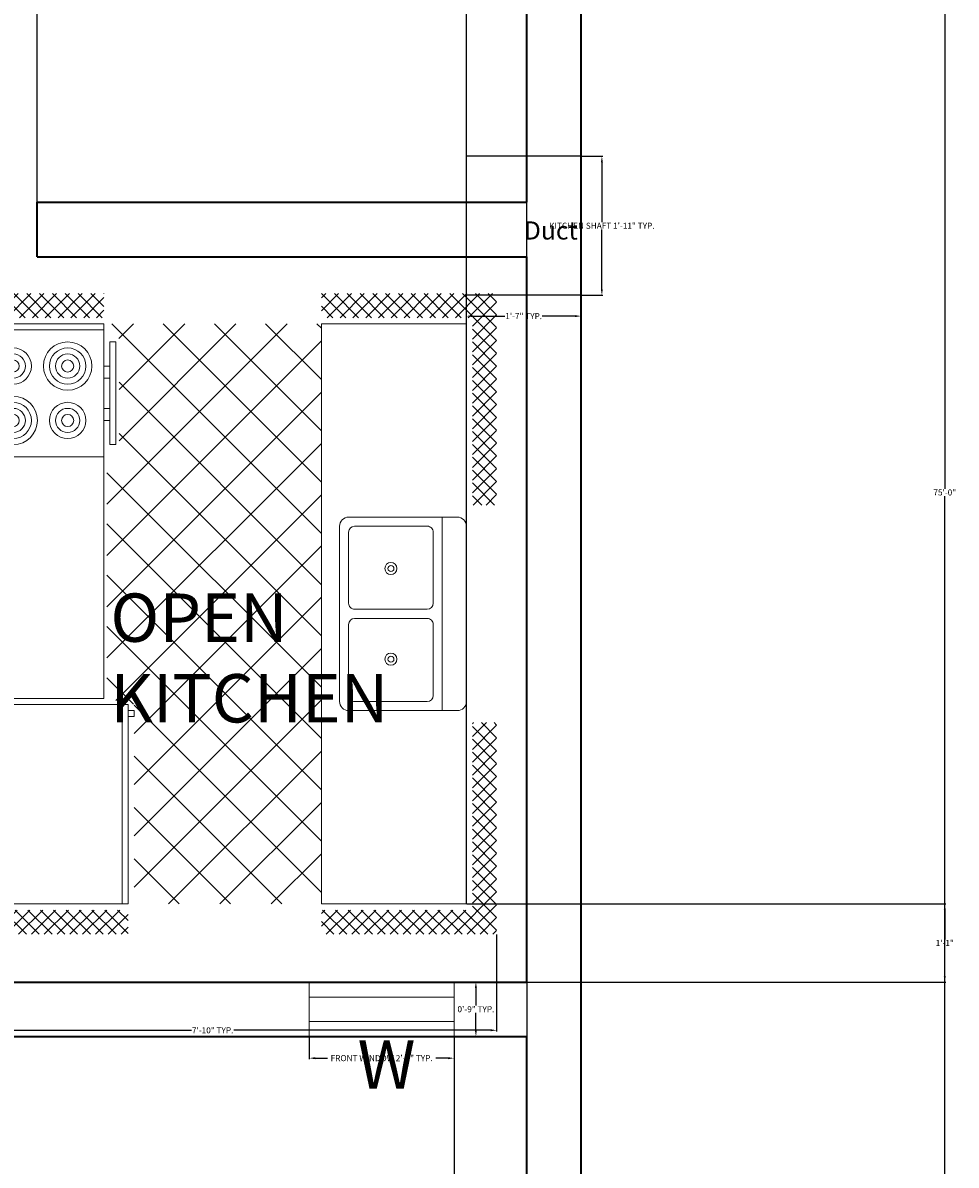
# Model space of a CAD drawing. Units: inches. Extents: x 371 to 1095, y -45 to 1219.
# Tile 12 of 18: x 940 to 1095, y 421 to 610. Entities that reach past the tile are written whole.
import ezdxf

# ---------------------------------------------------------------- set-up
doc = ezdxf.new("R2010")
doc.units = ezdxf.units.IN
doc.header["$MEASUREMENT"] = 0
for name, color, linetype, lineweight in [('A-ANNO-DIMS', 2, 'Continuous', 18), ('A-ANNO-TEXT', 7, 'Continuous', 18), ('A-AREA-IDEN', 7, 'Continuous', 18), ('A-FLOR-FIXT', 9, 'Continuous', 18), ('A-FLOR-SHFT', 7, 'Continuous', 25), ('A-GLAZ', 4, 'Continuous', 18), ('A-WALL', 40, 'Continuous', 35), ('C-SITE-WALL', 40, 'Continuous', 35)]:
    doc.layers.add(name, color=color, linetype=linetype, lineweight=lineweight)
doc.styles.get("Standard").update_dxf_attribs({"font": 'arial.ttf'})
doc.dimstyles.get("Standard").update_dxf_attribs({"dimtxt": 1, "dimasz": 1, "dimexe": 0.18, "dimexo": 0.0625, "dimgap": 0.09, "dimtad": 0, "dimtih": 1, "dimtoh": 1, "dimdec": 0, "dimzin": 0, "dimdsep": 46, "dimlunit": 3, "dimtxsty": 'Standard', "dimcen": 0.09, "dimadec": 0, "dimazin": 0, "dimtfac": 1, "dimtdec": 0, "dimtofl": 0, "dimtmove": 0, "dimatfit": 3, "dimfxl": 1, "dimtolj": 1, "dimtzin": 0, "dimarcsym": 0})

# ---------------------------------------------------------------- blocks, each defined once
blk = doc.blocks.new('Kitchen Layout - 7 x 8 ft')
for p, q in [((-5, 81.32), (2.68, 89)), ((-5, 83.44), (0.56, 89)), ((-5, 85.56), (-1.56, 89)), ((-5, 87.68), (-3.68, 89)), ((-1, 84.97), (-5, 88.97)), ((1.09, 85), (-2.91, 89)), ((3.21, 85), (-0.79, 89)), ((0.81, 85), (4.81, 89)), ((5.34, 85), (1.34, 89)), ((2.93, 85), (6.93, 89)), ((7.46, 85), (3.46, 89)), ((5.05, 85), (9.05, 89)), ((9.58, 85), (5.58, 89)), ((7.17, 85), (11.17, 89)), ((11.7, 85), (7.7, 89)), ((9.29, 85), (13.29, 89)), ((13.82, 85), (9.82, 89)), ((11.41, 85), (15.41, 89)), ((15.94, 85), (11.94, 89)), ((13.53, 85), (17.53, 89)), ((18.06, 85), (14.06, 89)), ((15.65, 85), (19.65, 89)), ((20.18, 85), (16.18, 89)), ((17.78, 85), (21.78, 89)), ((22.31, 85), (18.31, 89)), ((19.9, 85), (23.9, 89)), ((24.43, 85), (20.43, 89)), ((22.02, 85), (26.02, 89)), ((26.55, 85), (22.55, 89)), ((24.14, 85), (28.14, 89)), ((28.67, 85), (24.67, 89)), ((26.26, 85), (30.26, 89)), ((30.79, 85), (26.79, 89)), ((28.38, 85), (32.38, 89)), ((32.91, 85), (28.91, 89)), ((30.5, 85), (34.5, 89)), ((35.03, 85), (31.03, 89)), ((32.63, 85), (36.63, 89)), ((37.16, 85), (33.16, 89)), ((34.75, 85), (38.75, 89)), ((39.28, 85), (35.28, 89)), ((36.87, 85), (40.87, 89)), ((41.4, 85), (37.4, 89)), ((38.99, 85), (42.99, 89)), ((43.52, 85), (39.52, 89)), ((41.11, 85), (45.11, 89)), ((45.64, 85), (41.64, 89)), ((43.23, 85), (47.23, 89)), ((47.76, 85), (43.76, 89)), ((45.35, 85), (49.35, 89)), ((49.88, 85), (45.88, 89)), ((47.47, 85), (51.47, 89)), ((52, 85), (48, 89)), ((49.6, 85), (53.6, 89)), ((54.13, 85), (50.13, 89)), ((51.72, 85), (55.72, 89)), ((56.25, 85), (52.25, 89)), ((53.84, 85), (57.84, 89)), ((58.37, 85), (54.37, 89)), ((55.96, 85), (59.96, 89)), ((60.49, 85), (56.49, 89)), ((58.08, 85), (62.08, 89)), ((62.61, 85), (58.61, 89)), ((60.2, 85), (64.2, 89)), ((64.73, 85), (60.73, 89)), ((62.32, 85), (66.32, 89)), ((66.85, 85), (62.85, 89)), ((64.45, 85), (68.45, 89)), ((68.97, 85), (64.97, 89)), ((66.57, 85), (70.57, 89)), ((71.1, 85), (67.1, 89)), ((68.69, 85), (72.69, 89)), ((73.22, 85), (69.22, 89)), ((70.81, 85), (74.81, 89)), ((75.34, 85), (71.34, 89)), ((72.93, 85), (76.93, 89)), ((77.46, 85), (73.46, 89)), ((75.05, 85), (79.05, 89)), ((79.58, 85), (75.58, 89)), ((77.17, 85), (81.17, 89)), ((81.7, 85), (77.7, 89)), ((79.29, 85), (83.29, 89)), ((83.82, 85), (79.82, 89)), ((81.42, 85), (85.42, 89)), ((85.95, 85), (81.95, 89)), ((83.54, 85), (87.54, 89)), ((88.07, 85), (84.07, 89)), ((85.66, 85), (89.66, 89)), ((90.19, 85), (86.19, 89)), ((87.78, 85), (91.78, 89)), ((92.31, 85), (88.31, 89)), ((89.9, 85), (93.9, 89)), ((94.43, 85), (90.43, 89)), ((92.02, 85), (96.02, 89)), ((96.55, 85), (92.55, 89)), ((94.14, 85), (98.14, 89)), ((101, 82.67), (94.67, 89)), ((96.27, 85), (100.27, 89)), ((101, 84.79), (96.79, 89)), ((101, 86.92), (98.92, 89)), ((97, 83.61), (101, 87.61)), ((-1, 82.85), (-5, 86.85)), ((97, 81.49), (101, 85.49)), ((-1, 80.73), (-5, 84.73)), ((-5, 79.19), (-1, 83.19)), ((34, 84), (96, 84)), ((34, 60), (34, 84)), ((96, 84), (96, 60)), ((101, 80.55), (97, 84.55)), ((97, 79.37), (101, 83.37)), ((-1, 78.61), (-5, 82.61)), ((101, 78.43), (97, 82.43)), ((-5, 77.07), (-1, 81.07)), ((-1, 76.49), (-5, 80.49)), ((74, 81), (95, 81)), ((97, 77.25), (101, 81.25)), ((101, 76.31), (97, 80.31)), ((-5, 74.95), (-1, 78.95)), ((-1, 74.36), (-5, 78.36)), ((97, 75.13), (101, 79.13)), ((101, 74.19), (97, 78.19)), ((-5, 72.83), (-1, 76.83)), ((-1, 72.24), (-5, 76.24)), ((97, 73.01), (101, 77.01)), ((101, 72.07), (97, 76.07)), ((-5, 70.71), (-1, 74.71)), ((-1, 70.12), (-5, 74.12)), ((97, 70.89), (101, 74.89)), ((101, 69.95), (97, 73.95)), ((-5, 68.59), (-1, 72.59)), ((-1, 68), (-5, 72)), ((97, 68.76), (101, 72.76)), ((101, 67.82), (97, 71.82)), ((-5, 66.47), (-1, 70.47)), ((97, 66.64), (101, 70.64)), ((-1, 65.88), (-5, 69.88)), ((-5, 64.35), (-1, 68.35)), ((101, 65.7), (97, 69.7)), ((97, 64.52), (101, 68.52)), ((-1, 63.76), (-5, 67.76)), ((-5, 62.22), (-1, 66.22)), ((101, 63.58), (97, 67.58)), ((97, 62.4), (101, 66.4)), ((-1, 61.64), (-5, 65.64)), ((101, 61.46), (97, 65.46)), ((97, 60.28), (101, 64.28)), ((-5, 60.1), (-1, 64.1)), ((-1, 59.52), (-5, 63.52)), ((100.34, 60), (97, 63.34)), ((-5, 57.98), (-1, 61.98)), ((-1, 57.39), (-5, 61.39)), ((98.22, 60), (97, 61.22)), ((98.84, 60), (101, 62.16)), ((-1.73, 56), (-5, 59.27)), ((-4.86, 56), (-1, 59.86)), ((10.4, 24), (45.9, 59.5)), ((18.88, 24), (54.38, 59.5)), ((27.37, 24), (62.87, 59.5)), ((33.03, 55.11), (37.41, 59.5)), ((96, 60), (34, 60)), ((35.85, 24), (71.35, 59.5)), ((76.2, 24), (40.7, 59.5)), ((84.68, 24), (49.18, 59.5)), ((93.17, 24), (57.67, 59.5)), ((61.31, 24), (96, 58.69)), ((96, 29.65), (66.15, 59.5)), ((80, 60), (80, 59)), ((82, 59), (82, 60)), ((87, 59), (87, 60)), ((89, 60), (89, 59)), ((100.96, 60), (101, 60.04)), ((-3.85, 56), (-5, 57.15)), ((-2.74, 56), (-1, 57.74)), ((0, 57), (33, 57)), ((67.71, 24), (33.68, 58.04)), ((44.34, 24), (77.84, 57.5)), ((52.82, 24), (86.32, 57.5)), ((96, 38.14), (76.64, 57.5)), ((96, 46.63), (85.13, 57.5)), ((96, 55.11), (93.57, 57.54)), ((0, 30.57), (24.43, 55)), ((0, 39.06), (15.94, 55)), ((0, 47.54), (7.46, 55)), ((1.91, 24), (32.91, 55)), ((33.77, 24), (2.77, 55)), ((42.26, 24), (11.26, 55)), ((50.74, 24), (19.74, 55)), ((59.23, 24), (28.23, 55)), ((31, 55), (31, 56)), ((32, 55), (31, 55)), ((32, 56), (32, 55)), ((25.29, 24), (0, 49.29)), ((69.79, 24), (96, 50.21)), ((78.28, 24), (96, 41.72)), ((16.8, 24), (0, 40.8)), ((8.32, 24), (0, 32.32)), ((86.76, 24), (96, 33.24)), ((95.25, 24), (96, 24.75)), ((-5, 21.92), (-2.92, 24)), ((-5, 19.8), (-1, 23.8)), ((-1, 19.21), (-5, 23.21)), ((-1, 21.33), (-3.67, 24)), ((-1, 23.45), (-1.55, 24)), ((0, 24), (96, 24)), ((0, 0), (0, 24)), ((96, 24), (96, 0)), ((97, 22.1), (98.9, 24)), ((97, 19.97), (101, 23.97)), ((101, 19.03), (97, 23.03)), ((101, 21.16), (98.16, 24)), ((101, 23.28), (100.28, 24)), ((-5, 17.68), (-1, 21.68)), ((-1, 17.09), (-5, 21.09)), ((97, 17.85), (101, 21.85)), ((101, 16.91), (97, 20.91)), ((-5, 15.55), (-1, 19.55)), ((-1, 14.97), (-5, 18.97)), ((97, 15.73), (101, 19.73)), ((-5, 13.43), (-1, 17.43)), ((47.25, 6.5), (47.25, 18.5)), ((48.75, 18.5), (48.75, 6.5)), ((101, 14.79), (97, 18.79)), ((97, 13.61), (101, 17.61)), ((-1, 12.85), (-5, 16.85)), ((-5, 11.31), (-1, 15.31)), ((101, 12.67), (97, 16.67)), ((97, 11.49), (101, 15.49)), ((-1, 10.73), (-5, 14.73)), ((101, 10.55), (97, 14.55)), ((97, 9.37), (101, 13.37)), ((-5, 9.19), (-1, 13.19)), ((-1, 8.6), (-5, 12.6)), ((101, 8.43), (97, 12.43)), ((-5, 7.07), (-1, 11.07)), ((-1, 6.48), (-5, 10.48)), ((97, 7.25), (101, 11.25)), ((101, 6.31), (97, 10.31)), ((-5, 4.95), (-1, 8.95)), ((-1, 4.36), (-5, 8.36)), ((97, 5.12), (101, 9.12)), ((101, 4.18), (97, 8.18)), ((-5, 2.83), (-1, 6.83)), ((-1, 2.24), (-5, 6.24)), ((97, 3), (101, 7)), ((101, 2.06), (97, 6.06)), ((-5, 0.71), (-1, 4.71)), ((-1, 0.12), (-5, 4.12)), ((64, 4), (32, 4)), ((97, 0.88), (101, 4.88)), ((101, -0.06), (97, 3.94)), ((-5, -1.42), (-1, 2.58)), ((2, -5), (-5, 2)), ((93.24, -5), (101, 2.76)), ((-5, -3.54), (-1, 0.46)), ((96, 0), (0, 0)), ((95.36, -5), (101, 0.64)), ((101, -2.18), (97, 1.82)), ((-0.12, -5), (-5, -0.12)), ((-4.34, -5), (-0.34, -1)), ((-2.22, -5), (1.78, -1)), ((-0.1, -5), (3.9, -1)), ((4.12, -5), (0.12, -1)), ((2.02, -5), (6.02, -1)), ((6.24, -5), (2.24, -1)), ((4.14, -5), (8.14, -1)), ((8.36, -5), (4.36, -1)), ((6.27, -5), (10.27, -1)), ((10.48, -5), (6.48, -1)), ((8.39, -5), (12.39, -1)), ((12.6, -5), (8.6, -1)), ((10.51, -5), (14.51, -1)), ((14.73, -5), (10.73, -1)), ((12.63, -5), (16.63, -1)), ((16.85, -5), (12.85, -1)), ((14.75, -5), (18.75, -1)), ((18.97, -5), (14.97, -1)), ((16.87, -5), (20.87, -1)), ((21.09, -5), (17.09, -1)), ((18.99, -5), (22.99, -1)), ((23.21, -5), (19.21, -1)), ((21.11, -5), (25.11, -1)), ((25.33, -5), (21.33, -1)), ((23.24, -5), (27.24, -1)), ((27.45, -5), (23.45, -1)), ((25.36, -5), (29.36, -1)), ((29.57, -5), (25.57, -1)), ((30, -3.3), (27.7, -1)), ((30, -1.18), (29.82, -1)), ((66, -2.54), (67.54, -1)), ((66, -4.66), (69.66, -1)), ((69.88, -5), (66, -1.12)), ((67.78, -5), (71.78, -1)), ((72, -5), (68, -1)), ((69.9, -5), (73.9, -1)), ((74.12, -5), (70.12, -1)), ((72.03, -5), (76.03, -1)), ((76.24, -5), (72.24, -1)), ((74.15, -5), (78.15, -1)), ((78.36, -5), (74.36, -1)), ((76.27, -5), (80.27, -1)), ((80.49, -5), (76.49, -1)), ((78.39, -5), (82.39, -1)), ((82.61, -5), (78.61, -1)), ((80.51, -5), (84.51, -1)), ((84.73, -5), (80.73, -1)), ((82.63, -5), (86.63, -1)), ((86.85, -5), (82.85, -1)), ((84.75, -5), (88.75, -1)), ((88.97, -5), (84.97, -1)), ((86.88, -5), (90.88, -1)), ((91.09, -5), (87.09, -1)), ((89, -5), (93, -1)), ((93.21, -5), (89.21, -1)), ((91.12, -5), (95.12, -1)), ((95.34, -5), (91.34, -1)), ((97.46, -5), (93.46, -1)), ((99.58, -5), (95.58, -1)), ((101, -4.3), (97, -0.3)), ((97.48, -5), (101, -1.48)), ((-2.25, -5), (-5, -2.25)), ((27.48, -5), (30, -2.48)), ((67.76, -5), (66, -3.24)), ((99.6, -5), (101, -3.6)), ((-4.37, -5), (-5, -4.37)), ((29.6, -5), (30, -4.6))]:
    blk.add_line(p, q)
for points in [[(0, 56), (0, 84), (33, 84), (33, 56)], [(74, 60), (74, 84), (95, 84), (95, 60)], [(76, 58), (76, 59), (93, 59), (93, 58)]]:
    blk.add_lwpolyline(points, close=True)
for points in [[(33.5, 21), (62.5, 21)], [(32, 1.5), (32, 19.5)], [(34.5, 19.5), (46.25, 19.5)], [(49.75, 19.5), (61.5, 19.5)], [(64, 19.5), (64, 1.5)], [(33.5, 6.5), (33.5, 18.5)], [(62.5, 18.5), (62.5, 6.5)], [(46.25, 5.5), (34.5, 5.5)], [(61.5, 5.5), (49.75, 5.5)], [(62.5, 0), (33.5, 0)]]:
    blk.add_lwpolyline(points)
for centre, radius in [((80, 75), 4), ((80, 75), 3), ((89, 75), 3), ((80, 75), 2), ((80, 75), 1), ((89, 75), 2), ((89, 75), 1), ((89, 66), 4), ((80, 66), 3), ((89, 66), 3), ((80, 66), 2), ((80, 66), 1), ((89, 66), 2), ((89, 66), 1), ((40.5, 12.5), 1), ((55.5, 12.5), 1), ((40.5, 12.5), 0.5), ((55.5, 12.5), 0.5)]:
    blk.add_circle(centre, radius)
for centre, radius, start, end in [((33.5, 19.5), 1.5, 90, 180), ((62.5, 19.5), 1.5, 0, 90), ((34.5, 18.5), 1, 90, 180), ((46.25, 18.5), 1, 0, 90), ((49.75, 18.5), 1, 90, 180), ((61.5, 18.5), 1, 0, 90), ((34.5, 6.5), 1, 180, 270), ((46.25, 6.5), 1, 270, 0), ((49.75, 6.5), 1, 180, 270), ((61.5, 6.5), 1, 270, 0), ((33.5, 1.5), 1.5, 180, 270), ((62.5, 1.5), 1.5, 270, 0)]:
    blk.add_arc(centre, radius, start, end)
blk = doc.blocks.new('WIN-24-FRONT')
for p, q in [((0, 6.5), (24, 6.5)), ((0, 2.5), (24, 2.5))]:
    blk.add_line(p, q)
blk.add_lwpolyline([(0, 0), (24, 0), (24, 9), (0, 9)], close=True)
blk = doc.blocks.new('SHAFT-KITCHEN')
for p, q in [((19, 23), (0, 23)), ((0, 23), (0, 0)), ((19, 0), (19, 23)), ((19, 0), (0, 0))]:
    blk.add_line(p, q)
blk = doc.blocks.new('*D37')
at = {"layer": 'A-ANNO-DIMS', "color": 0, "lineweight": -2, "transparency": 16777216}
for p, q in [((924.84, 458.88), (924.84, 442.86)), ((1018.84, 458.88), (1018.84, 442.86)), ((925.84, 443.04), (968.31, 443.04)), ((1017.84, 443.04), (975.36, 443.04))]:
    blk.add_line(p, q, dxfattribs=at)
at = {"layer": 'A-ANNO-DIMS', "color": 0, "transparency": 16777216}
for points in [[(925.84, 443.21), (925.84, 442.88), (924.84, 443.04)], [(1017.84, 443.21), (1017.84, 442.88), (1018.84, 443.04)]]:
    blk.add_solid(points, dxfattribs=at)
at = {"layer": 'Defpoints', "color": 0, "transparency": 16777216}
for p in [(924.84, 458.94), (1018.84, 458.94), (924.84, 443.04)]:
    blk.add_point(p, dxfattribs=at)
at = {"layer": 'A-ANNO-DIMS', "color": 0, "transparency": 16777216, "insert": (971.84, 443.04), "char_height": 1, "attachment_point": 5}
blk.add_mtext('\\A1;7\'-10" TYP.', dxfattribs=at)
blk = doc.blocks.new('*D44')
at = {"layer": 'A-ANNO-DIMS', "color": 0, "lineweight": -2, "transparency": 16777216}
for p, q in [((987.81, 441.96), (987.81, 438.25)), ((1011.81, 441.96), (1011.81, 438.25)), ((988.81, 438.43), (990.84, 438.43)), ((1010.81, 438.43), (1008.78, 438.43))]:
    blk.add_line(p, q, dxfattribs=at)
at = {"layer": 'A-ANNO-DIMS', "color": 0, "transparency": 16777216}
for points in [[(988.81, 438.59), (988.81, 438.26), (987.81, 438.43)], [(1010.81, 438.59), (1010.81, 438.26), (1011.81, 438.43)]]:
    blk.add_solid(points, dxfattribs=at)
at = {"layer": 'Defpoints', "color": 0, "transparency": 16777216}
for p in [(987.81, 442.03), (1011.81, 442.03), (1011.81, 438.43)]:
    blk.add_point(p, dxfattribs=at)
at = {"layer": 'A-ANNO-DIMS', "color": 0, "transparency": 16777216, "insert": (999.81, 438.43), "char_height": 1, "attachment_point": 5}
blk.add_mtext('\\A1;FRONT WINDOW 2\'-0" TYP.', dxfattribs=at)
blk = doc.blocks.new('*D45')
at = {"layer": 'A-ANNO-DIMS', "color": 0, "lineweight": -2, "transparency": 16777216}
for p, q in [((1011.87, 451.03), (1015.59, 451.03)), ((1015.41, 450.03), (1015.41, 447.13)), ((1015.41, 443.03), (1015.41, 445.92)), ((1011.87, 442.03), (1015.59, 442.03))]:
    blk.add_line(p, q, dxfattribs=at)
at = {"layer": 'A-ANNO-DIMS', "color": 0, "transparency": 16777216}
for points in [[(1015.24, 450.03), (1015.57, 450.03), (1015.41, 451.03)], [(1015.24, 443.03), (1015.57, 443.03), (1015.41, 442.03)]]:
    blk.add_solid(points, dxfattribs=at)
at = {"layer": 'Defpoints', "color": 0, "transparency": 16777216}
for p in [(1011.81, 451.03), (1015.41, 451.03), (1011.81, 442.03)]:
    blk.add_point(p, dxfattribs=at)
at = {"layer": 'A-ANNO-DIMS', "color": 0, "transparency": 16777216, "insert": (1015.41, 446.53), "char_height": 1, "attachment_point": 5}
blk.add_mtext('\\A1;0\'-9" TYP.', dxfattribs=at)
blk = doc.blocks.new('*D48')
at = {"layer": 'A-ANNO-DIMS', "color": 0, "lineweight": -2, "transparency": 16777216}
for p, q in [((1032.87, 587.65), (1036.44, 587.65)), ((1036.26, 586.65), (1036.26, 576.76)), ((1036.26, 565.65), (1036.26, 575.55)), ((1032.87, 564.65), (1036.44, 564.65))]:
    blk.add_line(p, q, dxfattribs=at)
at = {"layer": 'A-ANNO-DIMS', "color": 0, "transparency": 16777216}
for points in [[(1036.09, 586.65), (1036.42, 586.65), (1036.26, 587.65)], [(1036.09, 565.65), (1036.42, 565.65), (1036.26, 564.65)]]:
    blk.add_solid(points, dxfattribs=at)
at = {"layer": 'Defpoints', "color": 0, "transparency": 16777216}
for p in [(1032.81, 587.65), (1036.26, 587.65), (1032.81, 564.65)]:
    blk.add_point(p, dxfattribs=at)
at = {"layer": 'A-ANNO-DIMS', "color": 0, "transparency": 16777216, "insert": (1036.26, 576.15), "char_height": 1, "attachment_point": 5}
blk.add_mtext('\\A1;KITCHEN SHAFT 1\'-11" TYP.', dxfattribs=at)
blk = doc.blocks.new('*D49')
at = {"layer": 'A-ANNO-DIMS', "color": 0, "lineweight": -2, "transparency": 16777216}
for p, q in [((1013.81, 564.59), (1013.81, 561.02)), ((1032.81, 564.59), (1032.81, 561.02)), ((1014.81, 561.2), (1020.22, 561.2)), ((1031.81, 561.2), (1026.4, 561.2))]:
    blk.add_line(p, q, dxfattribs=at)
at = {"layer": 'A-ANNO-DIMS', "color": 0, "transparency": 16777216}
for points in [[(1014.81, 561.37), (1014.81, 561.04), (1013.81, 561.2)], [(1031.81, 561.37), (1031.81, 561.04), (1032.81, 561.2)]]:
    blk.add_solid(points, dxfattribs=at)
at = {"layer": 'Defpoints', "color": 0, "transparency": 16777216}
for p in [(1013.81, 564.65), (1032.81, 564.65), (1032.81, 561.2)]:
    blk.add_point(p, dxfattribs=at)
at = {"layer": 'A-ANNO-DIMS', "color": 0, "transparency": 16777216, "insert": (1023.31, 561.2), "char_height": 1, "attachment_point": 5}
blk.add_mtext('\\A1;1\'-7" TYP.', dxfattribs=at)
blk = doc.blocks.new('*D51')
at = {"layer": 'A-ANNO-DIMS', "color": 0, "lineweight": -2, "transparency": 16777216}
for p, q in [((1032.87, 982.03), (1093.19, 982.03)), ((1093.01, 981.03), (1093.01, 532.63)), ((1093.01, 83.03), (1093.01, 531.42)), ((1032.87, 82.03), (1093.19, 82.03))]:
    blk.add_line(p, q, dxfattribs=at)
at = {"layer": 'A-ANNO-DIMS', "color": 0, "transparency": 16777216}
for points in [[(1092.84, 981.03), (1093.17, 981.03), (1093.01, 982.03)], [(1092.84, 83.03), (1093.17, 83.03), (1093.01, 82.03)]]:
    blk.add_solid(points, dxfattribs=at)
at = {"layer": 'Defpoints', "color": 0, "transparency": 16777216}
for p in [(1032.81, 982.03), (1093.01, 982.03), (1032.81, 82.03)]:
    blk.add_point(p, dxfattribs=at)
at = {"layer": 'A-ANNO-DIMS', "color": 0, "transparency": 16777216, "insert": (1093.01, 532.03), "char_height": 1, "attachment_point": 5}
blk.add_mtext('\\A1;75\'-0"', dxfattribs=at)
blk = doc.blocks.new('*D62')
at = {"layer": 'A-ANNO-DIMS', "color": 0, "lineweight": -2, "transparency": 16777216}
for p, q in [((1023.81, 450.96), (1023.81, -43.83)), ((1011.81, 441.96), (1011.81, -43.83)), ((1012.81, -43.65), (1016.44, -43.65)), ((1022.81, -43.65), (1019.18, -43.65))]:
    blk.add_line(p, q, dxfattribs=at)
at = {"layer": 'A-ANNO-DIMS', "color": 0, "transparency": 16777216}
for points in [[(1012.81, -43.48), (1012.81, -43.82), (1011.81, -43.65)], [(1022.81, -43.48), (1022.81, -43.82), (1023.81, -43.65)]]:
    blk.add_solid(points, dxfattribs=at)
at = {"layer": 'Defpoints', "color": 0, "transparency": 16777216}
for p in [(1023.81, 451.03), (1011.81, 442.03), (1023.81, -43.65)]:
    blk.add_point(p, dxfattribs=at)
at = {"layer": 'A-ANNO-DIMS', "color": 0, "transparency": 16777216, "insert": (1017.81, -43.65), "char_height": 1, "attachment_point": 5}
blk.add_mtext('\\A1;1\'-0"', dxfattribs=at)
blk = doc.blocks.new('*D63')
at = {"layer": 'A-ANNO-DIMS', "color": 0, "lineweight": -2, "transparency": 16777216}
for p, q in [((942.81, 580.09), (942.81, 1093.41)), ((943.81, 1093.23), (981.89, 1093.23)), ((1022.81, 1093.23), (984.73, 1093.23)), ((1023.81, 580.09), (1023.81, 1093.41))]:
    blk.add_line(p, q, dxfattribs=at)
at = {"layer": 'A-ANNO-DIMS', "color": 0, "transparency": 16777216}
for points in [[(943.81, 1093.39), (943.81, 1093.06), (942.81, 1093.23)], [(1022.81, 1093.39), (1022.81, 1093.06), (1023.81, 1093.23)]]:
    blk.add_solid(points, dxfattribs=at)
at = {"layer": 'Defpoints', "color": 0, "transparency": 16777216}
for p in [(1023.81, 1093.23), (942.81, 580.03), (1023.81, 580.03)]:
    blk.add_point(p, dxfattribs=at)
at = {"layer": 'A-ANNO-DIMS', "color": 0, "transparency": 16777216, "insert": (983.31, 1093.23), "char_height": 1, "attachment_point": 5}
blk.add_mtext('\\A1;6\'-9"', dxfattribs=at)
blk = doc.blocks.new('*D64')
at = {"layer": 'A-ANNO-DIMS', "color": 0, "lineweight": -2, "transparency": 16777216}
for p, q in [((1013.84, 464.01), (1013.84, 1093.41)), ((1014.84, 1093.23), (1017.01, 1093.23)), ((1022.81, 1093.23), (1020.63, 1093.23)), ((1023.81, 451.09), (1023.81, 1093.41))]:
    blk.add_line(p, q, dxfattribs=at)
at = {"layer": 'A-ANNO-DIMS', "color": 0, "transparency": 16777216}
for points in [[(1014.84, 1093.39), (1014.84, 1093.06), (1013.84, 1093.23)], [(1022.81, 1093.39), (1022.81, 1093.06), (1023.81, 1093.23)]]:
    blk.add_solid(points, dxfattribs=at)
at = {"layer": 'Defpoints', "color": 0, "transparency": 16777216}
for p in [(1023.81, 1093.23), (1013.84, 463.94), (1023.81, 451.03)]:
    blk.add_point(p, dxfattribs=at)
at = {"layer": 'A-ANNO-DIMS', "color": 0, "transparency": 16777216, "insert": (1018.82, 1093.23), "char_height": 1, "attachment_point": 5}
blk.add_mtext('\\A1;0\'-10"', dxfattribs=at)
blk = doc.blocks.new('*D65')
at = {"layer": 'A-ANNO-DIMS', "color": 0, "lineweight": -2, "transparency": 16777216}
for p, q in [((1013.9, 463.94), (1093.19, 463.94)), ((1093.01, 462.94), (1093.01, 458.08)), ((1093.01, 452.03), (1093.01, 456.89)), ((1023.87, 451.03), (1093.19, 451.03))]:
    blk.add_line(p, q, dxfattribs=at)
at = {"layer": 'A-ANNO-DIMS', "color": 0, "transparency": 16777216}
for points in [[(1092.84, 462.94), (1093.17, 462.94), (1093.01, 463.94)], [(1092.84, 452.03), (1093.17, 452.03), (1093.01, 451.03)]]:
    blk.add_solid(points, dxfattribs=at)
at = {"layer": 'Defpoints', "color": 0, "transparency": 16777216}
for p in [(1013.84, 463.94), (1023.81, 451.03), (1093.01, 451.03)]:
    blk.add_point(p, dxfattribs=at)
at = {"layer": 'A-ANNO-DIMS', "color": 0, "transparency": 16777216, "insert": (1093.01, 457.48), "char_height": 1, "attachment_point": 5}
blk.add_mtext('\\A1;1\'-1"', dxfattribs=at)

msp = doc.modelspace()

# ---------------------------------------------------------------- linework, layer by layer
at = {"layer": 'A-WALL'}
for p, q in [((1032.81, 82.03), (1032.81, 982.03)), ((1023.81, 580.03), (1023.81, 796.03)), ((942.81, 580.03), (1023.81, 580.03)), ((942.81, 571.03), (942.81, 580.03)), ((942.81, 571.03), (1023.81, 571.03)), ((1023.81, 451.03), (1023.81, 571.03)), ((890.81, 451.03), (1023.81, 451.03)), ((891.01, 442.02), (1023.81, 442.02))]:
    msp.add_line(p, q, dxfattribs=at)
at = {"layer": 'C-SITE-WALL'}
msp.add_line((1023.81, 91.03), (1023.81, 442.02), dxfattribs=at)

# ---------------------------------------------------------------- block references
at = {"layer": 'A-FLOR-FIXT', "rotation": 89.99999999999999}
msp.add_blockref('Kitchen Layout - 7 x 8 ft', (1013.84, 463.94), dxfattribs=at)
at = {"layer": 'A-FLOR-SHFT'}
msp.add_blockref('SHAFT-KITCHEN', (1013.81, 564.65), dxfattribs=at)
at = {"layer": 'A-GLAZ'}
msp.add_blockref('WIN-24-FRONT', (987.81, 442.02), dxfattribs=at)

# ---------------------------------------------------------------- texts
at = {"layer": 'A-ANNO-TEXT', "insert": (995.82, 441.37), "char_height": 8, "attachment_point": 1}
msp.add_mtext_dynamic_manual_height_columns('W', width=17.4938, gutter_width=1, heights=[0], dxfattribs=at)
at = {"layer": 'A-AREA-IDEN', "attachment_point": 1}
for s, width, insert, char_height in [('Duct', 31.9108, (1023.34, 576.87), 3), ('OPEN KITCHEN ', 53.6318, (954.91, 515.31), 8)]:
    msp.add_mtext_dynamic_manual_height_columns(s, width=width, gutter_width=1, heights=[0], dxfattribs=dict(at, insert=insert, char_height=char_height))

# ---------------------------------------------------------------- dimensions: what is measured, and where the dimension line sits
at = {"layer": 'A-ANNO-DIMS'}
for base, p1, p2, picture, middle in [((1023.81, 1093.23), (942.81, 580.03), (1023.81, 580.03), '*D63', (983.31, 1093.23)), ((1023.81, 1093.23), (1013.84, 463.94), (1023.81, 451.03), '*D64', (1018.82, 1093.23)), ((1023.81, -43.65), (1011.81, 442.02), (1023.81, 451.03), '*D62', (1017.81, -43.65))]:
    dim = msp.add_linear_dim(base=base, p1=p1, p2=p2, dimstyle='Standard', override={"dimdec": 1, "dimlfac": 1, "dimrnd": 0, "dimzin": 1, "dimdsep": 46, "dimlunit": 4, "dimfrac": 2}, dxfattribs=at)
    dim.commit()
    dim.dimension.update_dxf_attribs({"geometry": picture, "text_midpoint": middle})
for base, p1, p2, picture, middle in [((1093.01, 982.03), (1032.81, 82.03), (1032.81, 982.03), '*D51', (1093.01, 532.03)), ((1093.01, 451.03), (1013.84, 463.94), (1023.81, 451.03), '*D65', (1093.01, 457.48))]:
    dim = msp.add_linear_dim(base=base, p1=p1, p2=p2, angle=90, dimstyle='Standard', override={"dimdec": 1, "dimlfac": 1, "dimrnd": 0, "dimzin": 1, "dimdsep": 46, "dimlunit": 4, "dimfrac": 2}, dxfattribs=at)
    dim.commit()
    dim.dimension.update_dxf_attribs({"geometry": picture, "text_midpoint": middle})
for base, p1, p2, angle, text, picture, middle in [((1036.26, 587.65), (1032.81, 564.65), (1032.81, 587.65), 90, 'KITCHEN SHAFT <> TYP.', '*D48', (1036.26, 576.15)), ((924.84, 443.04), (1018.84, 458.94), (924.84, 458.94), 180, '<> TYP.', '*D37', (971.84, 443.04)), ((1015.41, 451.03), (1011.81, 442.02), (1011.81, 451.03), 90, '<> TYP.', '*D45', (1015.41, 446.53))]:
    dim = msp.add_linear_dim(base=base, p1=p1, p2=p2, angle=angle, text=text, dimstyle='Standard', override={"dimdec": 1, "dimlfac": 1, "dimrnd": 0, "dimzin": 1, "dimdsep": 46, "dimlunit": 4, "dimfrac": 2}, dxfattribs=at)
    dim.commit()
    dim.dimension.update_dxf_attribs({"geometry": picture, "text_midpoint": middle})
for base, p1, p2, text, picture, middle in [((1032.81, 561.2), (1013.81, 564.65), (1032.81, 564.65), '<> TYP.', '*D49', (1023.31, 561.2)), ((1011.81, 438.43), (987.81, 442.02), (1011.81, 442.02), 'FRONT WINDOW <> TYP.', '*D44', (999.81, 438.43))]:
    dim = msp.add_linear_dim(base=base, p1=p1, p2=p2, text=text, dimstyle='Standard', override={"dimdec": 1, "dimlfac": 1, "dimrnd": 0, "dimzin": 1, "dimdsep": 46, "dimlunit": 4, "dimfrac": 2}, dxfattribs=at)
    dim.commit()
    dim.dimension.update_dxf_attribs({"geometry": picture, "text_midpoint": middle})

doc.saveas('drawing.dxf')
